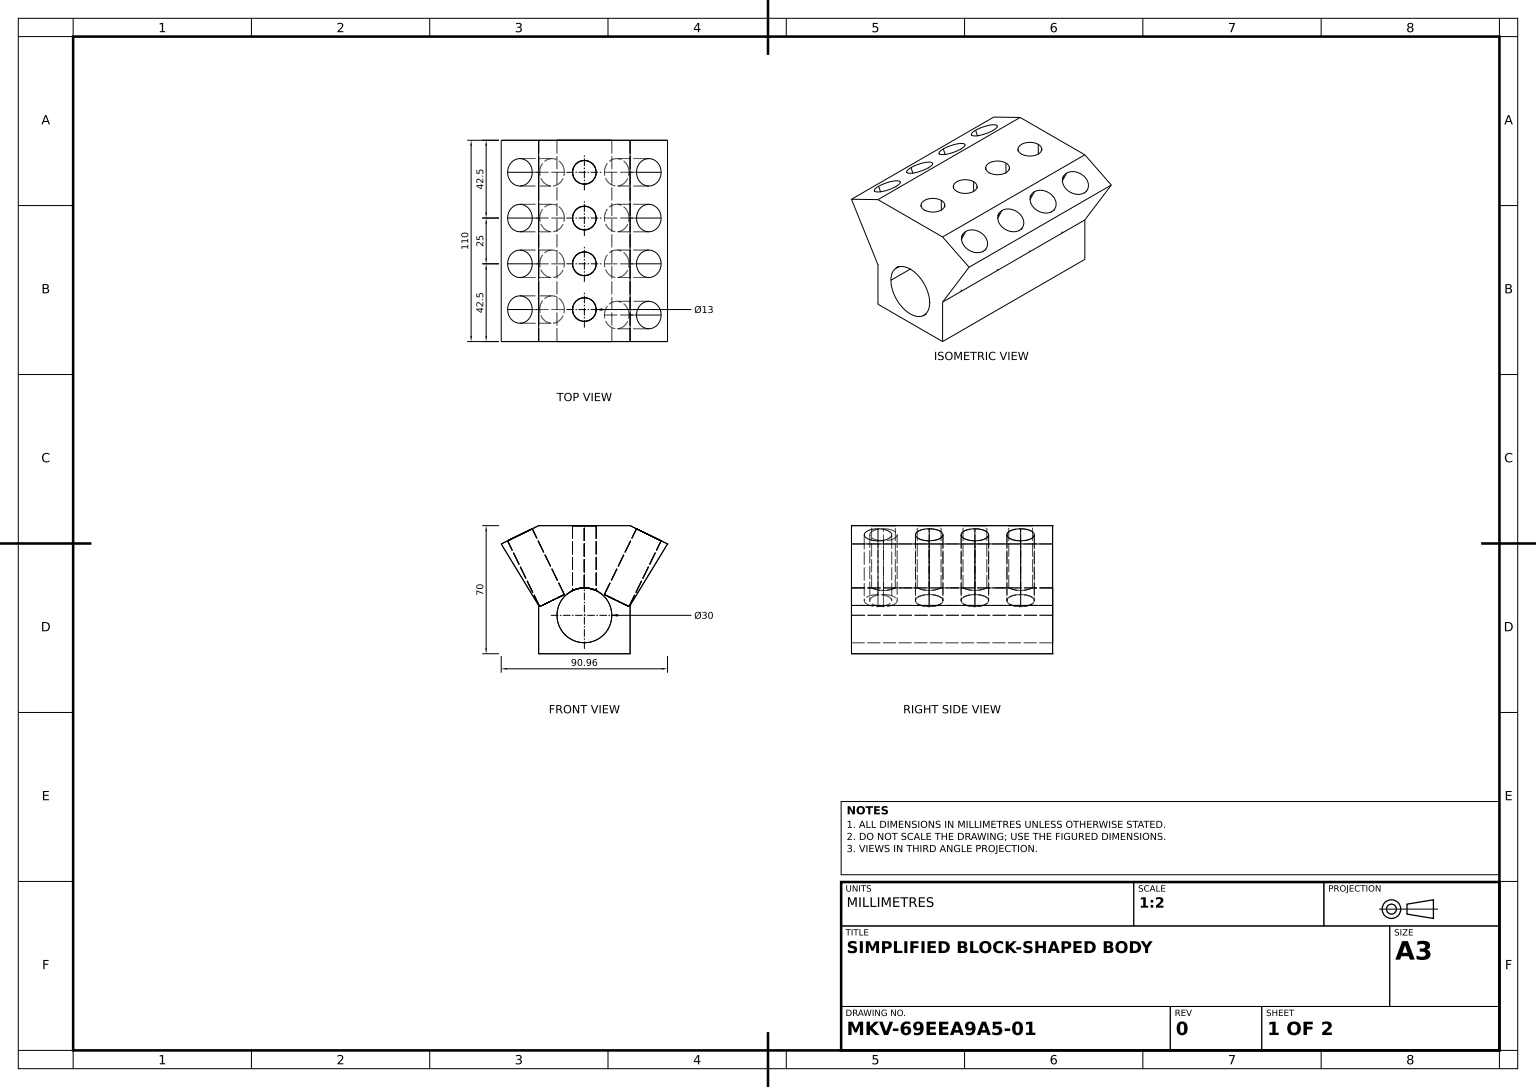
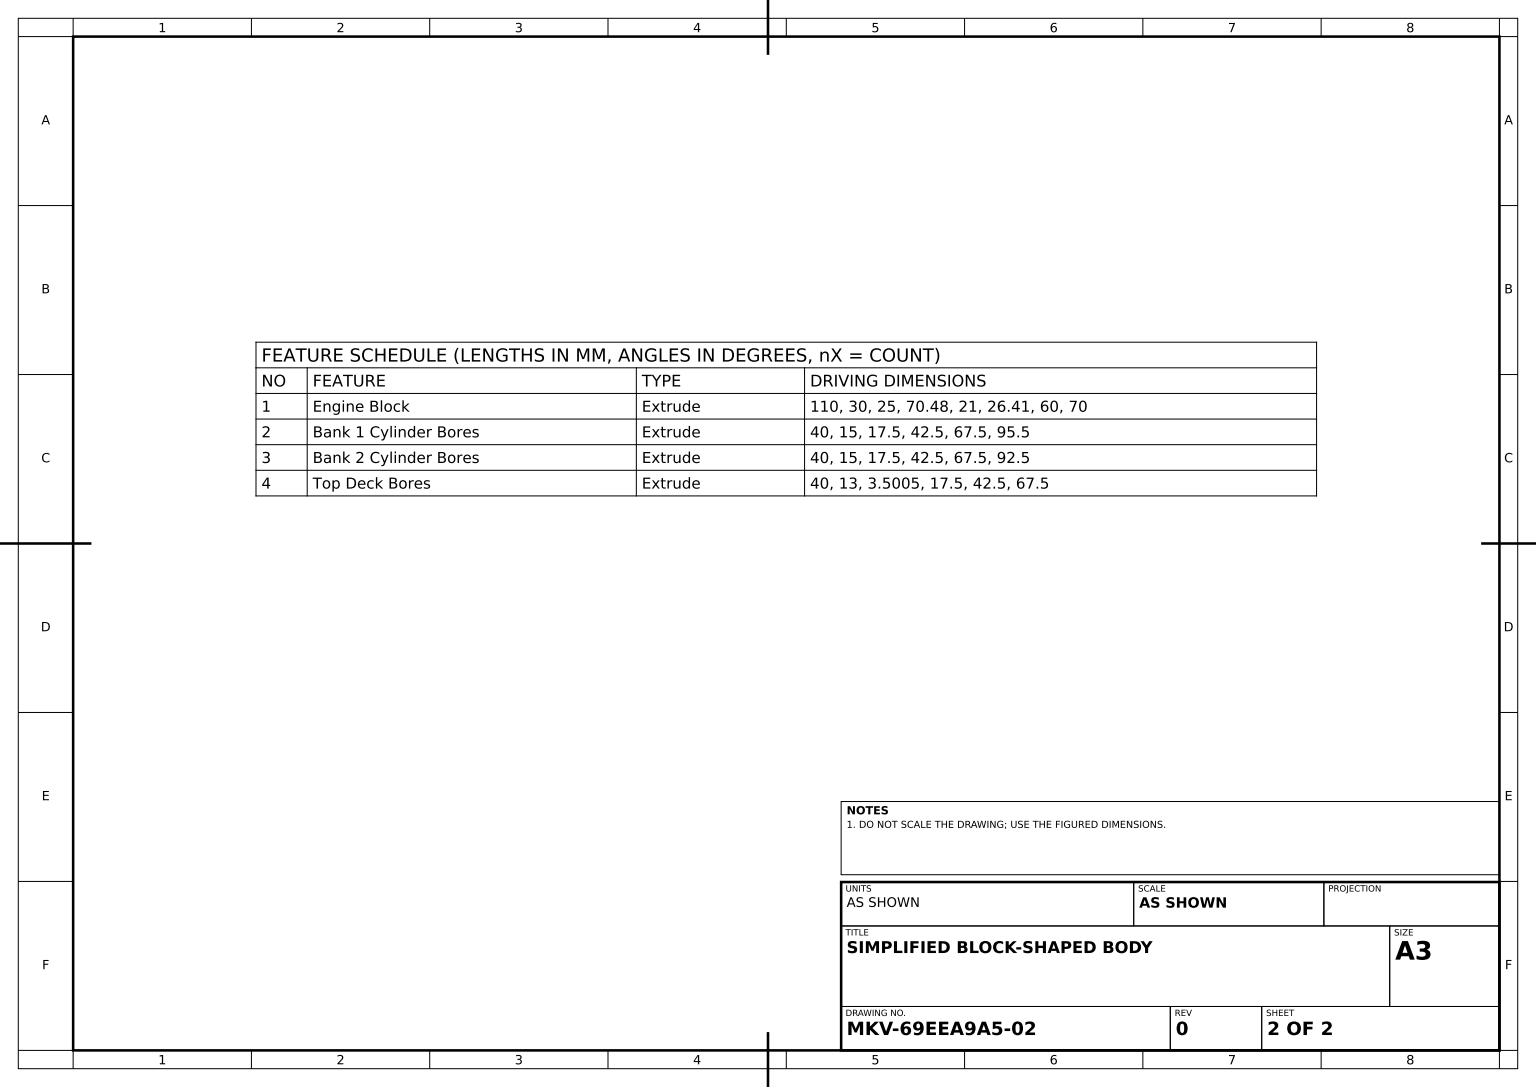
from build123d import *

# Parameters (mm, degrees)
BLOCK_PROFILE_SKETCH_R      = 15
ENGINE_BLOCK_DEPTH          = 110
BANK_1_CYLINDER_BORES_DEPTH = 40
BANK_2_BORES_SKETCH_R       = 7.5
BANK_2_CYLINDER_BORES_DEPTH = 40
TOP_DECK_BORES_SKETCH_R     = 6.5
TOP_DECK_BORES_DEPTH        = 40


with BuildPart() as part:
    # Block Profile Sketch → Engine Block (new body)
    with BuildSketch(Plane.XY):
        Polygon((-25, 0), (0, 0), (25, 0), (25, 26.41), (45.48, 60), (25, 70), (0, 70), (-25, 70), (-45.48, 60), (-25, 26.41), align=None)
        with Locations((0, 21)):
            Circle(BLOCK_PROFILE_SKETCH_R, mode=Mode.SUBTRACT)
    extrude(amount=-ENGINE_BLOCK_DEPTH)

    # Bank 1 Bores Sketch → Bank 1 Cylinder Bores (cut)
    with BuildSketch(Plane(origin=(32.412427151, 66.380650805, 0), x_dir=(0.8985997027642283, -0.43876938611534955, 0), z_dir=(0.4387693861153495, 0.8985997027642282, 0))):
        with BuildLine():
            ThreePointArc((3.146643428, 100), (-4.353356572, 92.5), (3.146643428, 85))
            Line((3.146643428, 85), (3.146643428, 92.5))
            Line((3.146643428, 92.5), (3.146643428, 100))
        make_face()
        with BuildLine():
            Line((3.146643428, 92.5), (3.146643428, 85))
            ThreePointArc((3.146643428, 85), (8.449944287, 87.196699141), (10.646643428, 92.5))
            Line((10.646643428, 92.5), (3.146643428, 92.5))
        make_face()
        with BuildLine():
            Line((3.146643428, 100), (3.146643428, 92.5))
            Line((3.146643428, 92.5), (10.646643428, 92.5))
            ThreePointArc((10.646643428, 92.5), (8.449944287, 97.803300859), (3.146643428, 100))
        make_face()
        with BuildLine():
            Line((3.146643428, 92.5), (3.146643428, 85))
            ThreePointArc((3.146643428, 85), (8.449944287, 87.196699141), (10.646643428, 92.5))
            Line((10.646643428, 92.5), (3.146643428, 92.5))
        make_face()
        with BuildLine():
            Line((3.146643428, 100), (3.146643428, 92.5))
            Line((3.146643428, 92.5), (10.646643428, 92.5))
            ThreePointArc((10.646643428, 92.5), (8.449944287, 97.803300859), (3.146643428, 100))
        make_face()
        with BuildLine():
            Line((3.146643428, 67.5), (3.146643428, 60))
            ThreePointArc((3.146643428, 60), (8.449944287, 62.196699141), (10.646643428, 67.5))
            Line((10.646643428, 67.5), (3.146643428, 67.5))
        make_face()
        with BuildLine():
            Line((3.146643428, 75), (3.146643428, 67.5))
            Line((3.146643428, 67.5), (10.646643428, 67.5))
            ThreePointArc((10.646643428, 67.5), (8.449944287, 72.803300859), (3.146643428, 75))
        make_face()
        with BuildLine():
            Line((3.146643428, 67.5), (3.146643428, 60))
            ThreePointArc((3.146643428, 60), (8.449944287, 62.196699141), (10.646643428, 67.5))
            Line((10.646643428, 67.5), (3.146643428, 67.5))
        make_face()
        with BuildLine():
            Line((3.146643428, 75), (3.146643428, 67.5))
            Line((3.146643428, 67.5), (10.646643428, 67.5))
            ThreePointArc((10.646643428, 67.5), (8.449944287, 72.803300859), (3.146643428, 75))
        make_face()
        with BuildLine():
            ThreePointArc((3.146643428, 75), (-4.353356572, 67.5), (3.146643428, 60))
            Line((3.146643428, 60), (3.146643428, 67.5))
            Line((3.146643428, 67.5), (3.146643428, 75))
        make_face()
        with BuildLine():
            ThreePointArc((3.146643428, 50), (-4.353356572, 42.5), (3.146643428, 35))
            Line((3.146643428, 35), (3.146643428, 42.5))
            Line((3.146643428, 42.5), (3.146643428, 50))
        make_face()
        with BuildLine():
            Line((3.146643428, 42.5), (3.146643428, 35))
            ThreePointArc((3.146643428, 35), (8.449944287, 37.196699141), (10.646643428, 42.5))
            Line((10.646643428, 42.5), (3.146643428, 42.5))
        make_face()
        with BuildLine():
            Line((3.146643428, 50), (3.146643428, 42.5))
            Line((3.146643428, 42.5), (10.646643428, 42.5))
            ThreePointArc((10.646643428, 42.5), (8.449944287, 47.803300859), (3.146643428, 50))
        make_face()
        with BuildLine():
            Line((3.146643428, 42.5), (3.146643428, 35))
            ThreePointArc((3.146643428, 35), (8.449944287, 37.196699141), (10.646643428, 42.5))
            Line((10.646643428, 42.5), (3.146643428, 42.5))
        make_face()
        with BuildLine():
            Line((3.146643428, 50), (3.146643428, 42.5))
            Line((3.146643428, 42.5), (10.646643428, 42.5))
            ThreePointArc((10.646643428, 42.5), (8.449944287, 47.803300859), (3.146643428, 50))
        make_face()
        with BuildLine():
            ThreePointArc((3.146643428, 22), (-4.353356572, 14.5), (3.146643428, 7))
            Line((3.146643428, 7), (3.146643428, 14.5))
            Line((3.146643428, 14.5), (3.146643428, 22))
        make_face()
        with BuildLine():
            Line((3.146643428, 14.5), (3.146643428, 7))
            ThreePointArc((3.146643428, 7), (8.449944287, 9.196699141), (10.646643428, 14.5))
            Line((10.646643428, 14.5), (3.146643428, 14.5))
        make_face()
        with BuildLine():
            Line((3.146643428, 22), (3.146643428, 14.5))
            Line((3.146643428, 14.5), (10.646643428, 14.5))
            ThreePointArc((10.646643428, 14.5), (8.449944287, 19.803300859), (3.146643428, 22))
        make_face()
        with BuildLine():
            Line((3.146643428, 14.5), (3.146643428, 7))
            ThreePointArc((3.146643428, 7), (8.449944287, 9.196699141), (10.646643428, 14.5))
            Line((10.646643428, 14.5), (3.146643428, 14.5))
        make_face()
        with BuildLine():
            Line((3.146643428, 22), (3.146643428, 14.5))
            Line((3.146643428, 14.5), (10.646643428, 14.5))
            ThreePointArc((10.646643428, 14.5), (8.449944287, 19.803300859), (3.146643428, 22))
        make_face()
    extrude(amount=-BANK_1_CYLINDER_BORES_DEPTH, mode=Mode.SUBTRACT)

    # Bank 2 Bores Sketch → Bank 2 Cylinder Bores (cut)
    with BuildSketch(Plane(origin=(-32.412427151, 66.380650805, 0), x_dir=(0.8985997027642294, 0.43876938611534716, 0), z_dir=(-0.4387693861153471, 0.8985997027642293, 0))):
        with Locations(Location((-3.146643428, 92.5, 0), (0, 0, 180))):
            Circle(BANK_2_BORES_SKETCH_R)
        with Locations(Location((-3.146643428, 67.5, 0), (0, 0, 180))):
            Circle(BANK_2_BORES_SKETCH_R)
        with Locations(Location((-3.146643428, 42.5, 0), (0, 0, 180))):
            Circle(BANK_2_BORES_SKETCH_R)
        with Locations(Location((-3.146643428, 17.5, 0), (0, 0, 180))):
            Circle(BANK_2_BORES_SKETCH_R)
    extrude(amount=-BANK_2_CYLINDER_BORES_DEPTH, mode=Mode.SUBTRACT)

    # Top Deck Bores Sketch → Top Deck Bores (cut)
    with BuildSketch(Plane(origin=(0, 70, 0), x_dir=(1, 0, 0), z_dir=(0, 1, 0))):
        with Locations(Location((0, 92.5, 0), (0, 0, 270))):
            Circle(TOP_DECK_BORES_SKETCH_R)
        with Locations(Location((0, 67.5, 0), (0, 0, 270))):
            Circle(TOP_DECK_BORES_SKETCH_R)
        with Locations(Location((0, 42.5, 0), (0, 0, 270))):
            Circle(TOP_DECK_BORES_SKETCH_R)
        with Locations(Location((0, 17.5, 0), (0, 0, 270))):
            Circle(TOP_DECK_BORES_SKETCH_R)
    extrude(amount=-TOP_DECK_BORES_DEPTH, mode=Mode.SUBTRACT)


solid = part.part
